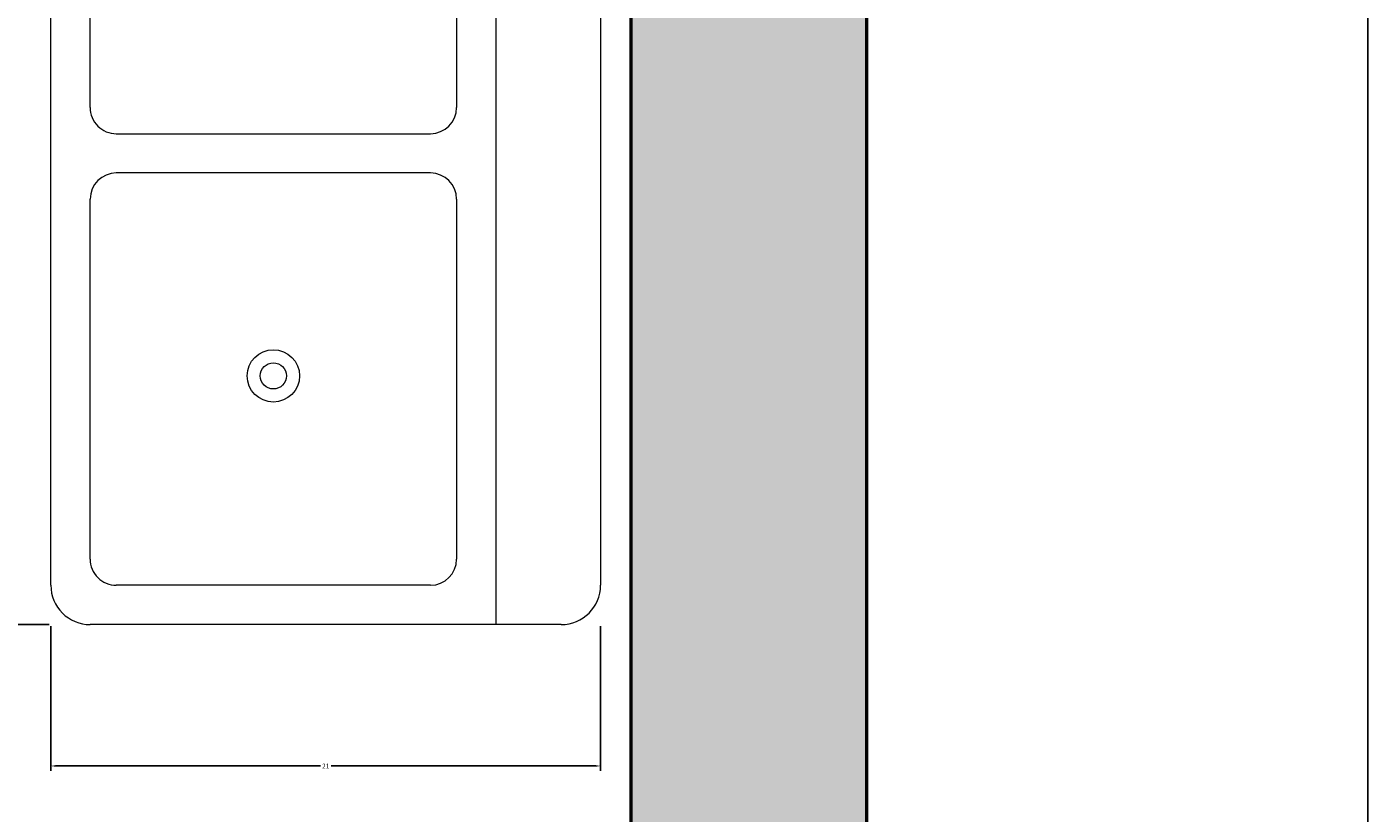
# Model space of a CAD drawing. Units: inches. Extents: x 2307 to 2544, y 2171 to 2540.
# Tile 38 of 52: x 2493 to 2544, y 2377 to 2407. Entities that reach past the tile are written whole.
import ezdxf

# ---------------------------------------------------------------- set-up
doc = ezdxf.new("R2010")
doc.units = ezdxf.units.IN
for name, color, linetype, lineweight in [('A-ANNO-DIMS', 2, 'Continuous', 18), ('A-FLOR-FIXT', 9, 'Continuous', 18), ('A-WALL', 7, 'Continuous', 50)]:
    doc.layers.add(name, color=color, linetype=linetype, lineweight=lineweight)
doc.layers.add('A-WALL-PATT', color=18, linetype='Continuous', lineweight=13, true_color=0x000000)
doc.styles.get("Standard").update_dxf_attribs({"font": 'arial.ttf'})
doc.dimstyles.get("Standard").update_dxf_attribs({"dimtxt": 0.18, "dimasz": 0.18, "dimexe": 0.18, "dimexo": 0.0625, "dimgap": 0.09, "dimtad": 0, "dimtih": 1, "dimtoh": 1, "dimdec": 4, "dimzin": 0, "dimdsep": 46, "dimtxsty": 'Standard', "dimcen": 0.09, "dimadec": 0, "dimazin": 0, "dimtfac": 1, "dimtdec": 4, "dimtofl": 0, "dimtmove": 0, "dimatfit": 3, "dimfxl": 1, "dimtolj": 1, "dimtzin": 0, "dimarcsym": 0})

# ---------------------------------------------------------------- blocks, each defined once
blk = doc.blocks.new('Sink-double - 36 in top')
for p, q in [((-18, -4), (18, -4)), ((-0.75, -18.5), (-0.75, -6.5)), ((0.75, -6.5), (0.75, -18.5))]:
    blk.add_line(p, q)
for points in [[(-16.5, 0), (16.5, 0)], [(-18, -19.5), (-18, -1.5)], [(18, -1.5), (18, -19.5)], [(-15.5, -5.5), (-1.75, -5.5)], [(1.75, -5.5), (15.5, -5.5)], [(-16.5, -18.5), (-16.5, -6.5)], [(16.5, -6.5), (16.5, -18.5)], [(-1.75, -19.5), (-15.5, -19.5)], [(15.5, -19.5), (1.75, -19.5)], [(16.5, -21), (-16.5, -21)]]:
    blk.add_lwpolyline(points)
for centre, radius in [((-8.5, -12.5), 1), ((8.5, -12.5), 1), ((-8.5, -12.5), 0.5), ((8.5, -12.5), 0.5)]:
    blk.add_circle(centre, radius)
for centre, radius, start, end in [((-16.5, -1.5), 1.5, 90, 180), ((16.5, -1.5), 1.5, 0, 90), ((-15.5, -6.5), 1, 90, 180), ((-1.75, -6.5), 1, 0, 90), ((1.75, -6.5), 1, 90, 180), ((15.5, -6.5), 1, 0, 90), ((-15.5, -18.5), 1, 180, 270), ((-1.75, -18.5), 1, 270, 0), ((1.75, -18.5), 1, 180, 270), ((15.5, -18.5), 1, 270, 0), ((-16.5, -19.5), 1.5, 180, 270), ((16.5, -19.5), 1.5, 270, 0)]:
    blk.add_arc(centre, radius, start, end)
blk = doc.blocks.new('*D32')
at = {"layer": 'A-ANNO-DIMS', "color": 0, "lineweight": -2, "transparency": 16777216}
for p, q in [((2493.473, 2420.657), (2487.956, 2420.657)), ((2488.136, 2420.477), (2488.136, 2402.84)), ((2488.136, 2384.837), (2488.136, 2402.474)), ((2493.473, 2384.657), (2487.956, 2384.657))]:
    blk.add_line(p, q, dxfattribs=at)
at = {"layer": 'A-ANNO-DIMS', "color": 0, "transparency": 16777216}
for points in [[(2488.106, 2420.477), (2488.166, 2420.477), (2488.136, 2420.657)], [(2488.106, 2384.837), (2488.166, 2384.837), (2488.136, 2384.657)]]:
    blk.add_solid(points, dxfattribs=at)
at = {"layer": 'Defpoints', "color": 0, "transparency": 16777216}
for p in [(2493.536, 2420.657), (2488.136, 2384.657), (2493.536, 2384.657)]:
    blk.add_point(p, dxfattribs=at)
at = {"layer": 'A-ANNO-DIMS', "color": 0, "transparency": 16777216, "insert": (2488.136, 2402.657), "char_height": 0.18, "attachment_point": 5}
blk.add_mtext('\\A1;DOUBLE SINK 36', dxfattribs=at)
blk = doc.blocks.new('*D33')
at = {"layer": 'A-ANNO-DIMS', "color": 0, "lineweight": -2, "transparency": 16777216}
for p, q in [((2493.536, 2384.595), (2493.536, 2379.077)), ((2514.536, 2384.595), (2514.536, 2379.077)), ((2493.716, 2379.257), (2503.833, 2379.257)), ((2514.356, 2379.257), (2504.239, 2379.257))]:
    blk.add_line(p, q, dxfattribs=at)
at = {"layer": 'A-ANNO-DIMS', "color": 0, "transparency": 16777216}
for points in [[(2493.716, 2379.287), (2493.716, 2379.227), (2493.536, 2379.257)], [(2514.356, 2379.287), (2514.356, 2379.227), (2514.536, 2379.257)]]:
    blk.add_solid(points, dxfattribs=at)
at = {"layer": 'Defpoints', "color": 0, "transparency": 16777216}
for p in [(2493.536, 2384.657), (2514.536, 2384.657), (2514.536, 2379.257)]:
    blk.add_point(p, dxfattribs=at)
at = {"layer": 'A-ANNO-DIMS', "color": 0, "transparency": 16777216, "insert": (2504.036, 2379.257), "char_height": 0.18, "attachment_point": 5}
blk.add_mtext('\\A1;21', dxfattribs=at)
blk = doc.blocks.new('*D37')
at = {"layer": 'A-ANNO-DIMS', "color": 0, "lineweight": -2, "transparency": 16777216}
for p, q in [((2524.758, 2520.51), (2544.026, 2520.51)), ((2543.846, 2520.33), (2543.846, 2355.692)), ((2543.846, 2190.69), (2543.846, 2355.328)), ((2524.758, 2190.51), (2544.026, 2190.51))]:
    blk.add_line(p, q, dxfattribs=at)
at = {"layer": 'A-ANNO-DIMS', "color": 0, "transparency": 16777216}
for points in [[(2543.816, 2520.33), (2543.876, 2520.33), (2543.846, 2520.51)], [(2543.816, 2190.69), (2543.876, 2190.69), (2543.846, 2190.51)]]:
    blk.add_solid(points, dxfattribs=at)
at = {"layer": 'Defpoints', "color": 0, "transparency": 16777216}
for p in [(2524.696, 2520.51), (2543.846, 2520.51), (2524.696, 2190.51)]:
    blk.add_point(p, dxfattribs=at)
at = {"layer": 'A-ANNO-DIMS', "color": 0, "transparency": 16777216, "insert": (2543.846, 2355.51), "char_height": 0.18, "attachment_point": 5}
blk.add_mtext('\\A1;330', dxfattribs=at)

msp = doc.modelspace()

# ---------------------------------------------------------------- hatches: boundary and pattern name
at = {"layer": 'A-WALL-PATT'}
h = msp.add_hatch(color=256, dxfattribs=at)
h.dxf.hatch_style = 1
h.paths.add_polyline_path([(2433.6935, 2199.5096), (2415.6423, 2199.5096), (2415.6423, 2190.5096), (2433.7832, 2190.5096)], flags=17)
h.paths.add_polyline_path([(2367.6423, 2199.5096), (2335.6958, 2199.5096), (2335.6958, 2307.3983), (2326.6958, 2307.3983), (2326.6958, 2190.5096), (2367.6423, 2190.5096)])
h.paths.add_polyline_path([(2524.6958, 2520.5096), (2496.7832, 2520.5096), (2496.7832, 2515.5149), (2472.7832, 2515.5149), (2472.7832, 2520.5096), (2415.4028, 2520.5096), (2415.4028, 2511.5096), (2451.6958, 2511.5096), (2451.6958, 2439.5096), (2451.6958, 2391.5096), (2445.6958, 2391.5096), (2445.6958, 2387.5096), (2455.6958, 2387.5096), (2455.6958, 2435.5096), (2461.6958, 2435.5096), (2461.6958, 2439.5096), (2455.6958, 2439.5096), (2455.6958, 2511.5096), (2515.6958, 2511.5096), (2515.6958, 2439.5096), (2491.6958, 2439.5096), (2491.6958, 2435.5096), (2515.6958, 2435.5096), (2515.6958, 2319.5096), (2451.6958, 2319.5096), (2451.6958, 2281.5096), (2481.6958, 2281.5096), (2481.6958, 2225.5096), (2485.6958, 2225.5096), (2485.6958, 2285.5096), (2455.6958, 2285.5096), (2455.6958, 2315.5096), (2515.6958, 2315.5096), (2515.6958, 2199.5096), (2469.6952, 2199.5096), (2469.785, 2190.5096), (2524.6958, 2190.5096)])

# ---------------------------------------------------------------- linework, layer by layer
at = {"layer": 'A-WALL'}
msp.add_line((2515.6958, 2435.5096), (2515.6958, 2319.5096), dxfattribs=at)
msp.add_lwpolyline([(2433.7832, 2190.5096), (2326.6958, 2190.5096), (2326.6958, 2520.5096), (2524.6958, 2520.5096), (2524.6958, 2190.5096), (2469.785, 2190.5096)], dxfattribs=at)

# ---------------------------------------------------------------- block references
at = {"layer": 'A-FLOR-FIXT', "rotation": 270}
msp.add_blockref('Sink-double - 36 in top', (2514.5356, 2402.6573), dxfattribs=at)

# ---------------------------------------------------------------- dimensions: what is measured, and where the dimension line sits
at = {"layer": 'A-ANNO-DIMS'}
dim = msp.add_linear_dim(base=(2543.8458, 2520.5096), p1=(2524.6958, 2190.5096), p2=(2524.6958, 2520.5096), angle=90, dimstyle='Standard', override={"dimdec": 0, "dimlfac": 1, "dimrnd": 0, "dimzin": 0, "dimdsep": 46, "dimlunit": 2}, dxfattribs=at)
dim.commit()
dim.dimension.update_dxf_attribs({"geometry": '*D37', "text_midpoint": (2543.8458, 2355.5096)})
dim = msp.add_linear_dim(base=(2488.1356, 2384.6573), p1=(2493.5356, 2420.6573), p2=(2493.5356, 2384.6573), angle=270, text='DOUBLE SINK <>', dimstyle='Standard', override={"dimdec": 0, "dimlfac": 1, "dimrnd": 0, "dimzin": 0, "dimdsep": 46, "dimlunit": 2}, dxfattribs=at)
dim.commit()
dim.dimension.update_dxf_attribs({"geometry": '*D32', "text_midpoint": (2488.1356, 2402.6573)})
dim = msp.add_linear_dim(base=(2514.5356, 2379.2573), p1=(2493.5356, 2384.6573), p2=(2514.5356, 2384.6573), dimstyle='Standard', override={"dimdec": 0, "dimlfac": 1, "dimrnd": 0, "dimzin": 0, "dimdsep": 46, "dimlunit": 2}, dxfattribs=at)
dim.commit()
dim.dimension.update_dxf_attribs({"geometry": '*D33', "text_midpoint": (2504.0356, 2379.2573)})

doc.saveas('drawing.dxf')
